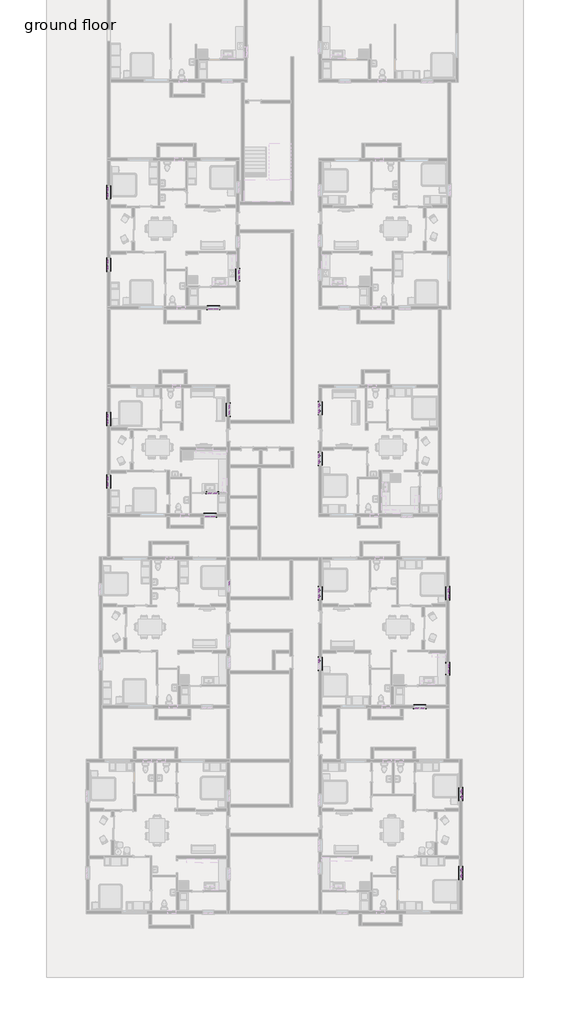
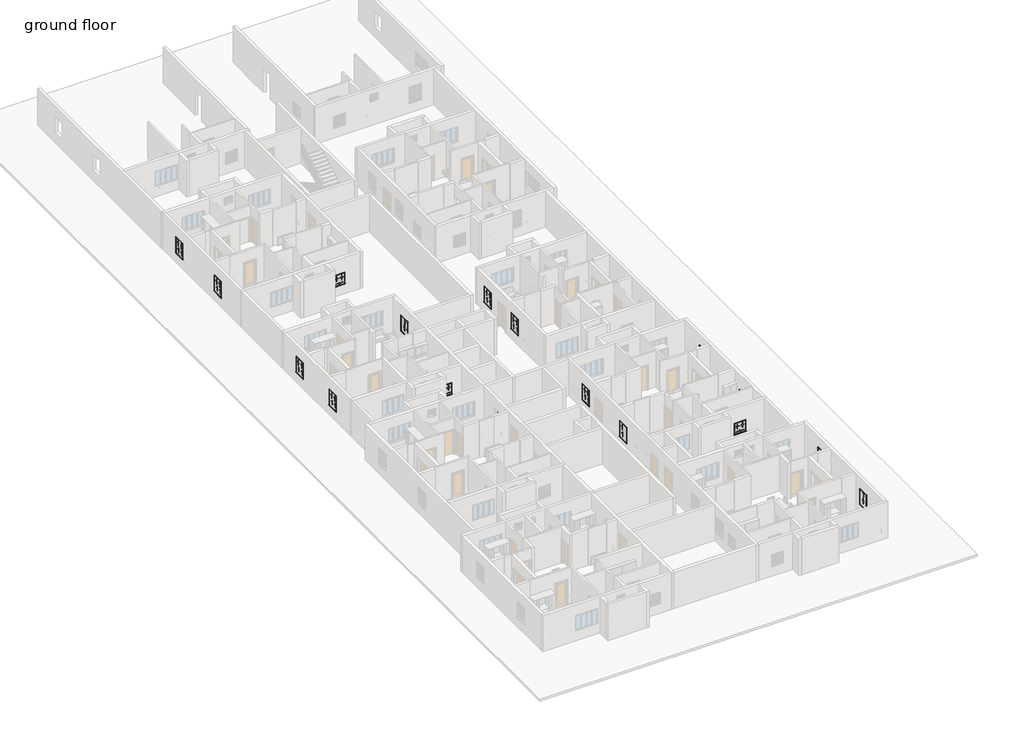
# One storey, part 15 of 16: 102 proxies.
"""IFC4 building model written with IfcOpenShell, lengths in millimetres."""

from ifc_helpers import new_model, si_unit, origin, place, context, project, spatial, transform, mapped, element, save
from components import muntin_pattern_2x2_muntin_pattern_2x2_cd1db81d, muntin_pattern_2x2_muntin_pattern_2x2_7c797e2d, muntin_pattern_2x2_muntin_pattern_2x2_78ce0566, muntin_pattern_2x2_muntin_pattern_2x2_27bf4e5b, muntin_pattern_2x2_muntin_pattern_2x2_8320156c, trim_window_exterior_flat_with_sill_fadbc092, trim_window_exterior_flat_with_sill_41619996, trim_window_interior_flat_picture_frame_db6fc9b7, trim_window_interior_flat_picture_frame_51c85655

model = new_model("IFC4")

# Units and contexts
model_context = context("Model", 3, world=origin())
ifc_project = project(units=[si_unit("LENGTHUNIT", "METRE", prefix="MILLI")], contexts=[model_context])

# Site, building, storey
site = spatial("IfcSite", under=ifc_project)
building = spatial("IfcBuilding", under=site)
storey = spatial("IfcBuildingStorey", under=building, Name="ground floor", Elevation=609.6)

# Proxies
placement = place(None, origin())
muntin_pattern_2x2_muntin_pattern_2x2_shape = muntin_pattern_2x2_muntin_pattern_2x2_cd1db81d(model_context)
element("IfcBuildingElementProxy", 1, Name="Muntin Pattern_2x2 : Muntin Pattern_2x2", ObjectType="Muntin Pattern_2x2 : Muntin Pattern_2x2", at=placement, inside=storey, context=model_context, shape_type="MappedRepresentation", body=[
    mapped(muntin_pattern_2x2_muntin_pattern_2x2_shape, transform((59391.4562819, 13667.0713152, 2206.625), x_axis=(0.0, 1.0, 0.0), y_axis=(-1.0, 0.0, 0.0), z_axis=(0.0, 0.0, 1.0))),
])
element("IfcBuildingElementProxy", 2, Name="Muntin Pattern_2x2 : Muntin Pattern_2x2", ObjectType="Muntin Pattern_2x2 : Muntin Pattern_2x2", at=placement, inside=storey, context=model_context, shape_type="MappedRepresentation", body=[
    mapped(muntin_pattern_2x2_muntin_pattern_2x2_shape, transform((59435.9062819, 13667.0713152, 1600.2), x_axis=(0.0, 1.0, 0.0), y_axis=(-1.0, 0.0, 0.0), z_axis=(0.0, 0.0, 1.0))),
])
element("IfcBuildingElementProxy", 3, Name="Muntin Pattern_2x2 : Muntin Pattern_2x2", ObjectType="Muntin Pattern_2x2 : Muntin Pattern_2x2", at=placement, inside=storey, context=model_context, shape_type="MappedRepresentation", body=[
    mapped(muntin_pattern_2x2_muntin_pattern_2x2_shape, transform((59391.4562819, 9780.8713152, 2206.625), x_axis=(0.0, 1.0, 0.0), y_axis=(-1.0, 0.0, 0.0), z_axis=(0.0, 0.0, 1.0))),
])
element("IfcBuildingElementProxy", 4, Name="Muntin Pattern_2x2 : Muntin Pattern_2x2", ObjectType="Muntin Pattern_2x2 : Muntin Pattern_2x2", at=placement, inside=storey, context=model_context, shape_type="MappedRepresentation", body=[
    mapped(muntin_pattern_2x2_muntin_pattern_2x2_shape, transform((59435.9062819, 9780.8713152, 1600.2), x_axis=(0.0, 1.0, 0.0), y_axis=(-1.0, 0.0, 0.0), z_axis=(0.0, 0.0, 1.0))),
])
element("IfcBuildingElementProxy", 5, Name="Muntin Pattern_2x2 : Muntin Pattern_2x2", ObjectType="Muntin Pattern_2x2 : Muntin Pattern_2x2", at=placement, inside=storey, context=model_context, shape_type="MappedRepresentation", body=[
    mapped(muntin_pattern_2x2_muntin_pattern_2x2_shape, transform((69329.2062819, -993.7176164, 2206.625), x_axis=(0.0, -1.0, 0.0), y_axis=(1.0, 0.0, 0.0), z_axis=(0.0, 0.0, 1.0))),
])
element("IfcBuildingElementProxy", 6, Name="Muntin Pattern_2x2 : Muntin Pattern_2x2", ObjectType="Muntin Pattern_2x2 : Muntin Pattern_2x2", at=placement, inside=storey, context=model_context, shape_type="MappedRepresentation", body=[
    mapped(muntin_pattern_2x2_muntin_pattern_2x2_shape, transform((69284.7562819, -993.7176164, 1600.2), x_axis=(0.0, -1.0, 0.0), y_axis=(1.0, 0.0, 0.0), z_axis=(0.0, 0.0, 1.0))),
])
element("IfcBuildingElementProxy", 7, Name="Muntin Pattern_2x2 : Muntin Pattern_2x2", ObjectType="Muntin Pattern_2x2 : Muntin Pattern_2x2", at=placement, inside=storey, context=model_context, shape_type="MappedRepresentation", body=[
    mapped(muntin_pattern_2x2_muntin_pattern_2x2_shape, transform((59391.4562819, -5948.3051164, 2206.625), x_axis=(0.0, 1.0, 0.0), y_axis=(-1.0, 0.0, 0.0), z_axis=(0.0, 0.0, 1.0))),
])
element("IfcBuildingElementProxy", 8, Name="Muntin Pattern_2x2 : Muntin Pattern_2x2", ObjectType="Muntin Pattern_2x2 : Muntin Pattern_2x2", at=placement, inside=storey, context=model_context, shape_type="MappedRepresentation", body=[
    mapped(muntin_pattern_2x2_muntin_pattern_2x2_shape, transform((59435.9062819, -5948.3051164, 1600.2), x_axis=(0.0, 1.0, 0.0), y_axis=(-1.0, 0.0, 0.0), z_axis=(0.0, 0.0, 1.0))),
])
element("IfcBuildingElementProxy", 9, Name="Muntin Pattern_2x2 : Muntin Pattern_2x2", ObjectType="Muntin Pattern_2x2 : Muntin Pattern_2x2", at=placement, inside=storey, context=model_context, shape_type="MappedRepresentation", body=[
    mapped(muntin_pattern_2x2_muntin_pattern_2x2_shape, transform((70332.5062819, -22465.6221086, 2206.625), x_axis=(0.0, -1.0, 0.0), y_axis=(1.0, 0.0, 0.0), z_axis=(0.0, 0.0, 1.0))),
])
element("IfcBuildingElementProxy", 10, Name="Muntin Pattern_2x2 : Muntin Pattern_2x2", ObjectType="Muntin Pattern_2x2 : Muntin Pattern_2x2", at=placement, inside=storey, context=model_context, shape_type="MappedRepresentation", body=[
    mapped(muntin_pattern_2x2_muntin_pattern_2x2_shape, transform((70288.0562819, -22465.6221086, 1600.2), x_axis=(0.0, -1.0, 0.0), y_axis=(1.0, 0.0, 0.0), z_axis=(0.0, 0.0, 1.0))),
])
element("IfcBuildingElementProxy", 11, Name="Muntin Pattern_2x2 : Muntin Pattern_2x2", ObjectType="Muntin Pattern_2x2 : Muntin Pattern_2x2", at=placement, inside=storey, context=model_context, shape_type="MappedRepresentation", body=[
    mapped(muntin_pattern_2x2_muntin_pattern_2x2_shape, transform((70332.5062819, -16407.8428409, 2206.625), x_axis=(0.0, -1.0, 0.0), y_axis=(1.0, 0.0, 0.0), z_axis=(0.0, 0.0, 1.0))),
])
element("IfcBuildingElementProxy", 12, Name="Muntin Pattern_2x2 : Muntin Pattern_2x2", ObjectType="Muntin Pattern_2x2 : Muntin Pattern_2x2", at=placement, inside=storey, context=model_context, shape_type="MappedRepresentation", body=[
    mapped(muntin_pattern_2x2_muntin_pattern_2x2_shape, transform((70288.0562819, -16407.8428409, 1600.2), x_axis=(0.0, -1.0, 0.0), y_axis=(1.0, 0.0, 0.0), z_axis=(0.0, 0.0, 1.0))),
])
element("IfcBuildingElementProxy", 13, Name="Muntin Pattern_2x2 : Muntin Pattern_2x2", ObjectType="Muntin Pattern_2x2 : Muntin Pattern_2x2", at=placement, inside=storey, context=model_context, shape_type="MappedRepresentation", body=[
    mapped(muntin_pattern_2x2_muntin_pattern_2x2_shape, transform((59391.4562819, -538.1051164, 2206.625), x_axis=(0.0, 1.0, 0.0), y_axis=(-1.0, 0.0, 0.0), z_axis=(0.0, 0.0, 1.0))),
])
element("IfcBuildingElementProxy", 14, Name="Muntin Pattern_2x2 : Muntin Pattern_2x2", ObjectType="Muntin Pattern_2x2 : Muntin Pattern_2x2", at=placement, inside=storey, context=model_context, shape_type="MappedRepresentation", body=[
    mapped(muntin_pattern_2x2_muntin_pattern_2x2_shape, transform((59435.9062819, -538.1051164, 1600.2), x_axis=(0.0, 1.0, 0.0), y_axis=(-1.0, 0.0, 0.0), z_axis=(0.0, 0.0, 1.0))),
])
element("IfcBuildingElementProxy", 15, Name="Muntin Pattern_2x2 : Muntin Pattern_2x2", ObjectType="Muntin Pattern_2x2 : Muntin Pattern_2x2", at=placement, inside=storey, context=model_context, shape_type="MappedRepresentation", body=[
    mapped(muntin_pattern_2x2_muntin_pattern_2x2_shape, transform((43176.551243, 8028.2713152, 2206.625), x_axis=(0.0, 1.0, 0.0), y_axis=(-1.0, 0.0, 0.0), z_axis=(0.0, 0.0, 1.0))),
])
element("IfcBuildingElementProxy", 16, Name="Muntin Pattern_2x2 : Muntin Pattern_2x2", ObjectType="Muntin Pattern_2x2 : Muntin Pattern_2x2", at=placement, inside=storey, context=model_context, shape_type="MappedRepresentation", body=[
    mapped(muntin_pattern_2x2_muntin_pattern_2x2_shape, transform((43221.001243, 8028.2713152, 1600.2), x_axis=(0.0, 1.0, 0.0), y_axis=(-1.0, 0.0, 0.0), z_axis=(0.0, 0.0, 1.0))),
])
element("IfcBuildingElementProxy", 17, Name="Muntin Pattern_2x2 : Muntin Pattern_2x2", ObjectType="Muntin Pattern_2x2 : Muntin Pattern_2x2", at=placement, inside=storey, context=model_context, shape_type="MappedRepresentation", body=[
    mapped(muntin_pattern_2x2_muntin_pattern_2x2_shape, transform((52504.701243, 13090.5355393, 2206.625), x_axis=(0.0, -1.0, 0.0), y_axis=(1.0, 0.0, 0.0), z_axis=(0.0, 0.0, 1.0))),
])
element("IfcBuildingElementProxy", 18, Name="Muntin Pattern_2x2 : Muntin Pattern_2x2", ObjectType="Muntin Pattern_2x2 : Muntin Pattern_2x2", at=placement, inside=storey, context=model_context, shape_type="MappedRepresentation", body=[
    mapped(muntin_pattern_2x2_muntin_pattern_2x2_shape, transform((52460.251243, 13090.5355393, 1600.2), x_axis=(0.0, -1.0, 0.0), y_axis=(1.0, 0.0, 0.0), z_axis=(0.0, 0.0, 1.0))),
])
element("IfcBuildingElementProxy", 19, Name="Muntin Pattern_2x2 : Muntin Pattern_2x2", ObjectType="Muntin Pattern_2x2 : Muntin Pattern_2x2", at=placement, inside=storey, context=model_context, shape_type="MappedRepresentation", body=[
    mapped(muntin_pattern_2x2_muntin_pattern_2x2_shape, transform((43176.551243, 12828.8713152, 2206.625), x_axis=(0.0, 1.0, 0.0), y_axis=(-1.0, 0.0, 0.0), z_axis=(0.0, 0.0, 1.0))),
])
element("IfcBuildingElementProxy", 20, Name="Muntin Pattern_2x2 : Muntin Pattern_2x2", ObjectType="Muntin Pattern_2x2 : Muntin Pattern_2x2", at=placement, inside=storey, context=model_context, shape_type="MappedRepresentation", body=[
    mapped(muntin_pattern_2x2_muntin_pattern_2x2_shape, transform((43221.001243, 12828.8713152, 1600.2), x_axis=(0.0, 1.0, 0.0), y_axis=(-1.0, 0.0, 0.0), z_axis=(0.0, 0.0, 1.0))),
])
element("IfcBuildingElementProxy", 21, Name="Muntin Pattern_2x2 : Muntin Pattern_2x2", ObjectType="Muntin Pattern_2x2 : Muntin Pattern_2x2", at=placement, inside=storey, context=model_context, shape_type="MappedRepresentation", body=[
    mapped(muntin_pattern_2x2_muntin_pattern_2x2_shape, transform((43176.551243, 24665.2713152, 2206.625), x_axis=(0.0, 1.0, 0.0), y_axis=(-1.0, 0.0, 0.0), z_axis=(0.0, 0.0, 1.0))),
])
element("IfcBuildingElementProxy", 22, Name="Muntin Pattern_2x2 : Muntin Pattern_2x2", ObjectType="Muntin Pattern_2x2 : Muntin Pattern_2x2", at=placement, inside=storey, context=model_context, shape_type="MappedRepresentation", body=[
    mapped(muntin_pattern_2x2_muntin_pattern_2x2_shape, transform((43221.001243, 24665.2713152, 1600.2), x_axis=(0.0, 1.0, 0.0), y_axis=(-1.0, 0.0, 0.0), z_axis=(0.0, 0.0, 1.0))),
])
element("IfcBuildingElementProxy", 23, Name="Muntin Pattern_2x2 : Muntin Pattern_2x2", ObjectType="Muntin Pattern_2x2 : Muntin Pattern_2x2", at=placement, inside=storey, context=model_context, shape_type="MappedRepresentation", body=[
    mapped(muntin_pattern_2x2_muntin_pattern_2x2_shape, transform((43176.551243, 30227.8713152, 2206.625), x_axis=(0.0, 1.0, 0.0), y_axis=(-1.0, 0.0, 0.0), z_axis=(0.0, 0.0, 1.0))),
])
element("IfcBuildingElementProxy", 24, Name="Muntin Pattern_2x2 : Muntin Pattern_2x2", ObjectType="Muntin Pattern_2x2 : Muntin Pattern_2x2", at=placement, inside=storey, context=model_context, shape_type="MappedRepresentation", body=[
    mapped(muntin_pattern_2x2_muntin_pattern_2x2_shape, transform((43221.001243, 30227.8713152, 1600.2), x_axis=(0.0, 1.0, 0.0), y_axis=(-1.0, 0.0, 0.0), z_axis=(0.0, 0.0, 1.0))),
])
muntin_pattern_2x2_muntin_pattern_2x2_2_shape = muntin_pattern_2x2_muntin_pattern_2x2_7c797e2d(model_context)
element("IfcBuildingElementProxy", 25, Name="Muntin Pattern_2x2 : Muntin Pattern_2x2", ObjectType="Muntin Pattern_2x2 : Muntin Pattern_2x2", at=placement, inside=storey, context=model_context, shape_type="MappedRepresentation", body=[
    mapped(muntin_pattern_2x2_muntin_pattern_2x2_2_shape, transform((59391.4562819, 13211.4588152, 2206.625), x_axis=(0.0, -1.0, 0.0), y_axis=(1.0, 0.0, 0.0), z_axis=(0.0, 0.0, 1.0))),
])
element("IfcBuildingElementProxy", 26, Name="Muntin Pattern_2x2 : Muntin Pattern_2x2", ObjectType="Muntin Pattern_2x2 : Muntin Pattern_2x2", at=placement, inside=storey, context=model_context, shape_type="MappedRepresentation", body=[
    mapped(muntin_pattern_2x2_muntin_pattern_2x2_2_shape, transform((59435.9062819, 13211.4588152, 1600.2), x_axis=(0.0, -1.0, 0.0), y_axis=(1.0, 0.0, 0.0), z_axis=(0.0, 0.0, 1.0))),
])
element("IfcBuildingElementProxy", 27, Name="Muntin Pattern_2x2 : Muntin Pattern_2x2", ObjectType="Muntin Pattern_2x2 : Muntin Pattern_2x2", at=placement, inside=storey, context=model_context, shape_type="MappedRepresentation", body=[
    mapped(muntin_pattern_2x2_muntin_pattern_2x2_2_shape, transform((59391.4562819, 9325.2588152, 2206.625), x_axis=(0.0, -1.0, 0.0), y_axis=(1.0, 0.0, 0.0), z_axis=(0.0, 0.0, 1.0))),
])
element("IfcBuildingElementProxy", 28, Name="Muntin Pattern_2x2 : Muntin Pattern_2x2", ObjectType="Muntin Pattern_2x2 : Muntin Pattern_2x2", at=placement, inside=storey, context=model_context, shape_type="MappedRepresentation", body=[
    mapped(muntin_pattern_2x2_muntin_pattern_2x2_2_shape, transform((59435.9062819, 9325.2588152, 1600.2), x_axis=(0.0, -1.0, 0.0), y_axis=(1.0, 0.0, 0.0), z_axis=(0.0, 0.0, 1.0))),
])
element("IfcBuildingElementProxy", 29, Name="Muntin Pattern_2x2 : Muntin Pattern_2x2", ObjectType="Muntin Pattern_2x2 : Muntin Pattern_2x2", at=placement, inside=storey, context=model_context, shape_type="MappedRepresentation", body=[
    mapped(muntin_pattern_2x2_muntin_pattern_2x2_2_shape, transform((69329.2062819, -538.1051164, 2206.625), x_axis=(0.0, 1.0, 0.0), y_axis=(-1.0, 0.0, 0.0), z_axis=(0.0, 0.0, 1.0))),
])
element("IfcBuildingElementProxy", 30, Name="Muntin Pattern_2x2 : Muntin Pattern_2x2", ObjectType="Muntin Pattern_2x2 : Muntin Pattern_2x2", at=placement, inside=storey, context=model_context, shape_type="MappedRepresentation", body=[
    mapped(muntin_pattern_2x2_muntin_pattern_2x2_2_shape, transform((69284.7562819, -538.1051164, 1600.2), x_axis=(0.0, 1.0, 0.0), y_axis=(-1.0, 0.0, 0.0), z_axis=(0.0, 0.0, 1.0))),
])
element("IfcBuildingElementProxy", 31, Name="Muntin Pattern_2x2 : Muntin Pattern_2x2", ObjectType="Muntin Pattern_2x2 : Muntin Pattern_2x2", at=placement, inside=storey, context=model_context, shape_type="MappedRepresentation", body=[
    mapped(muntin_pattern_2x2_muntin_pattern_2x2_2_shape, transform((70332.5062819, -22010.0096086, 2206.625), x_axis=(0.0, 1.0, 0.0), y_axis=(-1.0, 0.0, 0.0), z_axis=(0.0, 0.0, 1.0))),
])
element("IfcBuildingElementProxy", 32, Name="Muntin Pattern_2x2 : Muntin Pattern_2x2", ObjectType="Muntin Pattern_2x2 : Muntin Pattern_2x2", at=placement, inside=storey, context=model_context, shape_type="MappedRepresentation", body=[
    mapped(muntin_pattern_2x2_muntin_pattern_2x2_2_shape, transform((70288.0562819, -22010.0096086, 1600.2), x_axis=(0.0, 1.0, 0.0), y_axis=(-1.0, 0.0, 0.0), z_axis=(0.0, 0.0, 1.0))),
])
element("IfcBuildingElementProxy", 33, Name="Muntin Pattern_2x2 : Muntin Pattern_2x2", ObjectType="Muntin Pattern_2x2 : Muntin Pattern_2x2", at=placement, inside=storey, context=model_context, shape_type="MappedRepresentation", body=[
    mapped(muntin_pattern_2x2_muntin_pattern_2x2_2_shape, transform((70332.5062819, -15952.2303409, 2206.625), x_axis=(0.0, 1.0, 0.0), y_axis=(-1.0, 0.0, 0.0), z_axis=(0.0, 0.0, 1.0))),
])
element("IfcBuildingElementProxy", 34, Name="Muntin Pattern_2x2 : Muntin Pattern_2x2", ObjectType="Muntin Pattern_2x2 : Muntin Pattern_2x2", at=placement, inside=storey, context=model_context, shape_type="MappedRepresentation", body=[
    mapped(muntin_pattern_2x2_muntin_pattern_2x2_2_shape, transform((70288.0562819, -15952.2303409, 1600.2), x_axis=(0.0, 1.0, 0.0), y_axis=(-1.0, 0.0, 0.0), z_axis=(0.0, 0.0, 1.0))),
])
element("IfcBuildingElementProxy", 35, Name="Muntin Pattern_2x2 : Muntin Pattern_2x2", ObjectType="Muntin Pattern_2x2 : Muntin Pattern_2x2", at=placement, inside=storey, context=model_context, shape_type="MappedRepresentation", body=[
    mapped(muntin_pattern_2x2_muntin_pattern_2x2_2_shape, transform((59391.4562819, -993.7176164, 2206.625), x_axis=(0.0, -1.0, 0.0), y_axis=(1.0, 0.0, 0.0), z_axis=(0.0, 0.0, 1.0))),
])
element("IfcBuildingElementProxy", 36, Name="Muntin Pattern_2x2 : Muntin Pattern_2x2", ObjectType="Muntin Pattern_2x2 : Muntin Pattern_2x2", at=placement, inside=storey, context=model_context, shape_type="MappedRepresentation", body=[
    mapped(muntin_pattern_2x2_muntin_pattern_2x2_2_shape, transform((59435.9062819, -993.7176164, 1600.2), x_axis=(0.0, -1.0, 0.0), y_axis=(1.0, 0.0, 0.0), z_axis=(0.0, 0.0, 1.0))),
])
element("IfcBuildingElementProxy", 37, Name="Muntin Pattern_2x2 : Muntin Pattern_2x2", ObjectType="Muntin Pattern_2x2 : Muntin Pattern_2x2", at=placement, inside=storey, context=model_context, shape_type="MappedRepresentation", body=[
    mapped(muntin_pattern_2x2_muntin_pattern_2x2_2_shape, transform((43176.551243, 7572.6588152, 2206.625), x_axis=(0.0, -1.0, 0.0), y_axis=(1.0, 0.0, 0.0), z_axis=(0.0, 0.0, 1.0))),
])
element("IfcBuildingElementProxy", 38, Name="Muntin Pattern_2x2 : Muntin Pattern_2x2", ObjectType="Muntin Pattern_2x2 : Muntin Pattern_2x2", at=placement, inside=storey, context=model_context, shape_type="MappedRepresentation", body=[
    mapped(muntin_pattern_2x2_muntin_pattern_2x2_2_shape, transform((43221.001243, 7572.6588152, 1600.2), x_axis=(0.0, -1.0, 0.0), y_axis=(1.0, 0.0, 0.0), z_axis=(0.0, 0.0, 1.0))),
])
element("IfcBuildingElementProxy", 39, Name="Muntin Pattern_2x2 : Muntin Pattern_2x2", ObjectType="Muntin Pattern_2x2 : Muntin Pattern_2x2", at=placement, inside=storey, context=model_context, shape_type="MappedRepresentation", body=[
    mapped(muntin_pattern_2x2_muntin_pattern_2x2_2_shape, transform((52504.701243, 13546.1480393, 2206.625), x_axis=(0.0, 1.0, 0.0), y_axis=(-1.0, 0.0, 0.0), z_axis=(0.0, 0.0, 1.0))),
])
element("IfcBuildingElementProxy", 40, Name="Muntin Pattern_2x2 : Muntin Pattern_2x2", ObjectType="Muntin Pattern_2x2 : Muntin Pattern_2x2", at=placement, inside=storey, context=model_context, shape_type="MappedRepresentation", body=[
    mapped(muntin_pattern_2x2_muntin_pattern_2x2_2_shape, transform((52460.251243, 13546.1480393, 1600.2), x_axis=(0.0, 1.0, 0.0), y_axis=(-1.0, 0.0, 0.0), z_axis=(0.0, 0.0, 1.0))),
])
element("IfcBuildingElementProxy", 41, Name="Muntin Pattern_2x2 : Muntin Pattern_2x2", ObjectType="Muntin Pattern_2x2 : Muntin Pattern_2x2", at=placement, inside=storey, context=model_context, shape_type="MappedRepresentation", body=[
    mapped(muntin_pattern_2x2_muntin_pattern_2x2_2_shape, transform((43176.551243, 12373.2588152, 2206.625), x_axis=(0.0, -1.0, 0.0), y_axis=(1.0, 0.0, 0.0), z_axis=(0.0, 0.0, 1.0))),
])
element("IfcBuildingElementProxy", 42, Name="Muntin Pattern_2x2 : Muntin Pattern_2x2", ObjectType="Muntin Pattern_2x2 : Muntin Pattern_2x2", at=placement, inside=storey, context=model_context, shape_type="MappedRepresentation", body=[
    mapped(muntin_pattern_2x2_muntin_pattern_2x2_2_shape, transform((43221.001243, 12373.2588152, 1600.2), x_axis=(0.0, -1.0, 0.0), y_axis=(1.0, 0.0, 0.0), z_axis=(0.0, 0.0, 1.0))),
])
element("IfcBuildingElementProxy", 43, Name="Muntin Pattern_2x2 : Muntin Pattern_2x2", ObjectType="Muntin Pattern_2x2 : Muntin Pattern_2x2", at=placement, inside=storey, context=model_context, shape_type="MappedRepresentation", body=[
    mapped(muntin_pattern_2x2_muntin_pattern_2x2_2_shape, transform((43176.551243, 24209.6588152, 2206.625), x_axis=(0.0, -1.0, 0.0), y_axis=(1.0, 0.0, 0.0), z_axis=(0.0, 0.0, 1.0))),
])
element("IfcBuildingElementProxy", 44, Name="Muntin Pattern_2x2 : Muntin Pattern_2x2", ObjectType="Muntin Pattern_2x2 : Muntin Pattern_2x2", at=placement, inside=storey, context=model_context, shape_type="MappedRepresentation", body=[
    mapped(muntin_pattern_2x2_muntin_pattern_2x2_2_shape, transform((43221.001243, 24209.6588152, 1600.2), x_axis=(0.0, -1.0, 0.0), y_axis=(1.0, 0.0, 0.0), z_axis=(0.0, 0.0, 1.0))),
])
element("IfcBuildingElementProxy", 45, Name="Muntin Pattern_2x2 : Muntin Pattern_2x2", ObjectType="Muntin Pattern_2x2 : Muntin Pattern_2x2", at=placement, inside=storey, context=model_context, shape_type="MappedRepresentation", body=[
    mapped(muntin_pattern_2x2_muntin_pattern_2x2_2_shape, transform((43176.551243, 29772.2588152, 2206.625), x_axis=(0.0, -1.0, 0.0), y_axis=(1.0, 0.0, 0.0), z_axis=(0.0, 0.0, 1.0))),
])
element("IfcBuildingElementProxy", 46, Name="Muntin Pattern_2x2 : Muntin Pattern_2x2", ObjectType="Muntin Pattern_2x2 : Muntin Pattern_2x2", at=placement, inside=storey, context=model_context, shape_type="MappedRepresentation", body=[
    mapped(muntin_pattern_2x2_muntin_pattern_2x2_2_shape, transform((43221.001243, 29772.2588152, 1600.2), x_axis=(0.0, -1.0, 0.0), y_axis=(1.0, 0.0, 0.0), z_axis=(0.0, 0.0, 1.0))),
])
element("IfcBuildingElementProxy", 47, Name="Muntin Pattern_2x2 : Muntin Pattern_2x2", ObjectType="Muntin Pattern_2x2 : Muntin Pattern_2x2", at=placement, inside=storey, context=model_context, shape_type="MappedRepresentation", body=[
    mapped(muntin_pattern_2x2_muntin_pattern_2x2_2_shape, transform((52504.701243, 2.9653185, 2206.625), x_axis=(0.0, 1.0, 0.0), y_axis=(-1.0, 0.0, 0.0), z_axis=(0.0, 0.0, 1.0))),
])
element("IfcBuildingElementProxy", 48, Name="Muntin Pattern_2x2 : Muntin Pattern_2x2", ObjectType="Muntin Pattern_2x2 : Muntin Pattern_2x2", at=placement, inside=storey, context=model_context, shape_type="MappedRepresentation", body=[
    mapped(muntin_pattern_2x2_muntin_pattern_2x2_2_shape, transform((52460.251243, 2.9653185, 1600.2), x_axis=(0.0, 1.0, 0.0), y_axis=(-1.0, 0.0, 0.0), z_axis=(0.0, 0.0, 1.0))),
])
muntin_pattern_2x2_muntin_pattern_2x2_3_shape = muntin_pattern_2x2_muntin_pattern_2x2_78ce0566(model_context)
element("IfcBuildingElementProxy", 49, Name="Muntin Pattern_2x2 : Muntin Pattern_2x2", ObjectType="Muntin Pattern_2x2 : Muntin Pattern_2x2", at=placement, inside=storey, context=model_context, shape_type="MappedRepresentation", body=[
    mapped(muntin_pattern_2x2_muntin_pattern_2x2_3_shape, transform((69354.6062819, -6345.9738664, 1898.65), x_axis=(0.0, -1.0, 0.0), y_axis=(1.0, 0.0, 0.0), z_axis=(0.0, 0.0, 1.0))),
])
element("IfcBuildingElementProxy", 50, Name="Muntin Pattern_2x2 : Muntin Pattern_2x2", ObjectType="Muntin Pattern_2x2 : Muntin Pattern_2x2", at=placement, inside=storey, context=model_context, shape_type="MappedRepresentation", body=[
    mapped(muntin_pattern_2x2_muntin_pattern_2x2_3_shape, transform((67322.6640239, -9591.2174723, 1898.65), x_axis=(-1.0, 0.0, 0.0), y_axis=(0.0, -1.0, 0.0), z_axis=(0.0, 0.0, 1.0))),
])
element("IfcBuildingElementProxy", 51, Name="Muntin Pattern_2x2 : Muntin Pattern_2x2", ObjectType="Muntin Pattern_2x2 : Muntin Pattern_2x2", at=placement, inside=storey, context=model_context, shape_type="MappedRepresentation", body=[
    mapped(muntin_pattern_2x2_muntin_pattern_2x2_3_shape, transform((51229.408333, 5101.5968163, 1898.65), x_axis=(-1.0, 0.0, 0.0), y_axis=(0.0, -1.0, 0.0), z_axis=(0.0, 0.0, 1.0))),
])
element("IfcBuildingElementProxy", 52, Name="Muntin Pattern_2x2 : Muntin Pattern_2x2", ObjectType="Muntin Pattern_2x2 : Muntin Pattern_2x2", at=placement, inside=storey, context=model_context, shape_type="MappedRepresentation", body=[
    mapped(muntin_pattern_2x2_muntin_pattern_2x2_3_shape, transform((51417.263743, 6895.5900652, 1898.65), x_axis=(-1.0, 0.0, 0.0), y_axis=(0.0, -1.0, 0.0), z_axis=(0.0, 0.0, 1.0))),
])
element("IfcBuildingElementProxy", 53, Name="Muntin Pattern_2x2 : Muntin Pattern_2x2", ObjectType="Muntin Pattern_2x2 : Muntin Pattern_2x2", at=placement, inside=storey, context=model_context, shape_type="MappedRepresentation", body=[
    mapped(muntin_pattern_2x2_muntin_pattern_2x2_3_shape, transform((51489.2925, 21030.5522014, 1898.65), x_axis=(-1.0, 0.0, 0.0), y_axis=(0.0, -1.0, 0.0), z_axis=(0.0, 0.0, 1.0))),
])
element("IfcBuildingElementProxy", 54, Name="Muntin Pattern_2x2 : Muntin Pattern_2x2", ObjectType="Muntin Pattern_2x2 : Muntin Pattern_2x2", at=placement, inside=storey, context=model_context, shape_type="MappedRepresentation", body=[
    mapped(muntin_pattern_2x2_muntin_pattern_2x2_3_shape, transform((53254.001243, 23886.6025652, 1898.65), x_axis=(0.0, -1.0, 0.0), y_axis=(1.0, 0.0, 0.0), z_axis=(0.0, 0.0, 1.0))),
])
muntin_pattern_2x2_muntin_pattern_2x2_4_shape = muntin_pattern_2x2_muntin_pattern_2x2_27bf4e5b(model_context)
element("IfcBuildingElementProxy", 55, Name="Muntin Pattern_2x2 : Muntin Pattern_2x2", ObjectType="Muntin Pattern_2x2 : Muntin Pattern_2x2", at=placement, inside=storey, context=model_context, shape_type="MappedRepresentation", body=[
    mapped(muntin_pattern_2x2_muntin_pattern_2x2_4_shape, transform((69354.6062819, -6774.5988664, 1898.65), x_axis=(0.0, 1.0, 0.0), y_axis=(-1.0, 0.0, 0.0), z_axis=(0.0, 0.0, 1.0))),
])
element("IfcBuildingElementProxy", 56, Name="Muntin Pattern_2x2 : Muntin Pattern_2x2", ObjectType="Muntin Pattern_2x2 : Muntin Pattern_2x2", at=placement, inside=storey, context=model_context, shape_type="MappedRepresentation", body=[
    mapped(muntin_pattern_2x2_muntin_pattern_2x2_4_shape, transform((66894.0390239, -9591.2174723, 1898.65), x_axis=(1.0, 0.0, 0.0), y_axis=(0.0, 1.0, 0.0), z_axis=(0.0, 0.0, 1.0))),
])
element("IfcBuildingElementProxy", 57, Name="Muntin Pattern_2x2 : Muntin Pattern_2x2", ObjectType="Muntin Pattern_2x2 : Muntin Pattern_2x2", at=placement, inside=storey, context=model_context, shape_type="MappedRepresentation", body=[
    mapped(muntin_pattern_2x2_muntin_pattern_2x2_4_shape, transform((50800.783333, 5101.5968163, 1898.65), x_axis=(1.0, 0.0, 0.0), y_axis=(0.0, 1.0, 0.0), z_axis=(0.0, 0.0, 1.0))),
])
element("IfcBuildingElementProxy", 58, Name="Muntin Pattern_2x2 : Muntin Pattern_2x2", ObjectType="Muntin Pattern_2x2 : Muntin Pattern_2x2", at=placement, inside=storey, context=model_context, shape_type="MappedRepresentation", body=[
    mapped(muntin_pattern_2x2_muntin_pattern_2x2_4_shape, transform((50988.638743, 6895.5900652, 1898.65), x_axis=(1.0, 0.0, 0.0), y_axis=(0.0, 1.0, 0.0), z_axis=(0.0, 0.0, 1.0))),
])
element("IfcBuildingElementProxy", 59, Name="Muntin Pattern_2x2 : Muntin Pattern_2x2", ObjectType="Muntin Pattern_2x2 : Muntin Pattern_2x2", at=placement, inside=storey, context=model_context, shape_type="MappedRepresentation", body=[
    mapped(muntin_pattern_2x2_muntin_pattern_2x2_4_shape, transform((51060.6675, 21030.5522014, 1898.65), x_axis=(1.0, 0.0, 0.0), y_axis=(0.0, 1.0, 0.0), z_axis=(0.0, 0.0, 1.0))),
])
element("IfcBuildingElementProxy", 60, Name="Muntin Pattern_2x2 : Muntin Pattern_2x2", ObjectType="Muntin Pattern_2x2 : Muntin Pattern_2x2", at=placement, inside=storey, context=model_context, shape_type="MappedRepresentation", body=[
    mapped(muntin_pattern_2x2_muntin_pattern_2x2_4_shape, transform((53254.001243, 23457.9775652, 1898.65), x_axis=(0.0, 1.0, 0.0), y_axis=(-1.0, 0.0, 0.0), z_axis=(0.0, 0.0, 1.0))),
])
muntin_pattern_2x2_muntin_pattern_2x2_5_shape = muntin_pattern_2x2_muntin_pattern_2x2_8320156c(model_context)
element("IfcBuildingElementProxy", 61, Name="Muntin Pattern_2x2 : Muntin Pattern_2x2", ObjectType="Muntin Pattern_2x2 : Muntin Pattern_2x2", at=placement, inside=storey, context=model_context, shape_type="MappedRepresentation", body=[
    mapped(muntin_pattern_2x2_muntin_pattern_2x2_5_shape, transform((69354.6062819, -6560.2863664, 1593.85), x_axis=(0.0, 1.0, 0.0), y_axis=(-1.0, 0.0, 0.0), z_axis=(0.0, 0.0, 1.0))),
])
element("IfcBuildingElementProxy", 62, Name="Muntin Pattern_2x2 : Muntin Pattern_2x2", ObjectType="Muntin Pattern_2x2 : Muntin Pattern_2x2", at=placement, inside=storey, context=model_context, shape_type="MappedRepresentation", body=[
    mapped(muntin_pattern_2x2_muntin_pattern_2x2_5_shape, transform((67108.3515239, -9591.2174723, 1593.85), x_axis=(1.0, 0.0, 0.0), y_axis=(0.0, 1.0, 0.0), z_axis=(0.0, 0.0, 1.0))),
])
element("IfcBuildingElementProxy", 63, Name="Muntin Pattern_2x2 : Muntin Pattern_2x2", ObjectType="Muntin Pattern_2x2 : Muntin Pattern_2x2", at=placement, inside=storey, context=model_context, shape_type="MappedRepresentation", body=[
    mapped(muntin_pattern_2x2_muntin_pattern_2x2_5_shape, transform((51015.095833, 5101.5968163, 1593.85), x_axis=(1.0, 0.0, 0.0), y_axis=(0.0, 1.0, 0.0), z_axis=(0.0, 0.0, 1.0))),
])
element("IfcBuildingElementProxy", 64, Name="Muntin Pattern_2x2 : Muntin Pattern_2x2", ObjectType="Muntin Pattern_2x2 : Muntin Pattern_2x2", at=placement, inside=storey, context=model_context, shape_type="MappedRepresentation", body=[
    mapped(muntin_pattern_2x2_muntin_pattern_2x2_5_shape, transform((51202.951243, 6895.5900652, 1593.85), x_axis=(1.0, 0.0, 0.0), y_axis=(0.0, 1.0, 0.0), z_axis=(0.0, 0.0, 1.0))),
])
element("IfcBuildingElementProxy", 65, Name="Muntin Pattern_2x2 : Muntin Pattern_2x2", ObjectType="Muntin Pattern_2x2 : Muntin Pattern_2x2", at=placement, inside=storey, context=model_context, shape_type="MappedRepresentation", body=[
    mapped(muntin_pattern_2x2_muntin_pattern_2x2_5_shape, transform((51274.98, 21030.5522014, 1593.85), x_axis=(1.0, 0.0, 0.0), y_axis=(0.0, 1.0, 0.0), z_axis=(0.0, 0.0, 1.0))),
])
element("IfcBuildingElementProxy", 66, Name="Muntin Pattern_2x2 : Muntin Pattern_2x2", ObjectType="Muntin Pattern_2x2 : Muntin Pattern_2x2", at=placement, inside=storey, context=model_context, shape_type="MappedRepresentation", body=[
    mapped(muntin_pattern_2x2_muntin_pattern_2x2_5_shape, transform((53254.001243, 23672.2900652, 1593.85), x_axis=(0.0, 1.0, 0.0), y_axis=(-1.0, 0.0, 0.0), z_axis=(0.0, 0.0, 1.0))),
])
trim_window_exterior_flat_with_sill_shape = trim_window_exterior_flat_with_sill_fadbc092(model_context)
element("IfcBuildingElementProxy", 67, Name="Trim-Window-Exterior-Flat : with Sill", ObjectType="Trim-Window-Exterior-Flat : with Sill", at=placement, inside=storey, context=model_context, shape_type="MappedRepresentation", body=[
    mapped(trim_window_exterior_flat_with_sill_shape, transform((59356.5312819, 13439.2650652, 2844.8), x_axis=(0.0, -1.0, 0.0), y_axis=(0.0, 0.0, 1.0), z_axis=(-1.0, 0.0, 0.0))),
])
element("IfcBuildingElementProxy", 68, Name="Trim-Window-Exterior-Flat : with Sill", ObjectType="Trim-Window-Exterior-Flat : with Sill", at=placement, inside=storey, context=model_context, shape_type="MappedRepresentation", body=[
    mapped(trim_window_exterior_flat_with_sill_shape, transform((59356.5312819, 9553.0650652, 2844.8), x_axis=(0.0, -1.0, 0.0), y_axis=(0.0, 0.0, 1.0), z_axis=(-1.0, 0.0, 0.0))),
])
element("IfcBuildingElementProxy", 69, Name="Trim-Window-Exterior-Flat : with Sill", ObjectType="Trim-Window-Exterior-Flat : with Sill", at=placement, inside=storey, context=model_context, shape_type="MappedRepresentation", body=[
    mapped(trim_window_exterior_flat_with_sill_shape, transform((69364.1312819, -765.9113664, 2844.8), x_axis=(0.0, 1.0, 0.0), y_axis=(0.0, 0.0, 1.0), z_axis=(1.0, 0.0, 0.0))),
])
element("IfcBuildingElementProxy", 70, Name="Trim-Window-Exterior-Flat : with Sill", ObjectType="Trim-Window-Exterior-Flat : with Sill", at=placement, inside=storey, context=model_context, shape_type="MappedRepresentation", body=[
    mapped(trim_window_exterior_flat_with_sill_shape, transform((59356.5312819, -6176.1113664, 2844.8), x_axis=(0.0, -1.0, 0.0), y_axis=(0.0, 0.0, 1.0), z_axis=(-1.0, 0.0, 0.0))),
])
element("IfcBuildingElementProxy", 71, Name="Trim-Window-Exterior-Flat : with Sill", ObjectType="Trim-Window-Exterior-Flat : with Sill", at=placement, inside=storey, context=model_context, shape_type="MappedRepresentation", body=[
    mapped(trim_window_exterior_flat_with_sill_shape, transform((70367.4312819, -22237.8158586, 2844.8), x_axis=(0.0, 1.0, 0.0), y_axis=(0.0, 0.0, 1.0), z_axis=(1.0, 0.0, 0.0))),
])
element("IfcBuildingElementProxy", 72, Name="Trim-Window-Exterior-Flat : with Sill", ObjectType="Trim-Window-Exterior-Flat : with Sill", at=placement, inside=storey, context=model_context, shape_type="MappedRepresentation", body=[
    mapped(trim_window_exterior_flat_with_sill_shape, transform((70367.4312819, -16180.0365909, 2844.8), x_axis=(0.0, 1.0, 0.0), y_axis=(0.0, 0.0, 1.0), z_axis=(1.0, 0.0, 0.0))),
])
element("IfcBuildingElementProxy", 73, Name="Trim-Window-Exterior-Flat : with Sill", ObjectType="Trim-Window-Exterior-Flat : with Sill", at=placement, inside=storey, context=model_context, shape_type="MappedRepresentation", body=[
    mapped(trim_window_exterior_flat_with_sill_shape, transform((59356.5312819, -765.9113664, 2844.8), x_axis=(0.0, -1.0, 0.0), y_axis=(0.0, 0.0, 1.0), z_axis=(-1.0, 0.0, 0.0))),
])
element("IfcBuildingElementProxy", 74, Name="Trim-Window-Exterior-Flat : with Sill", ObjectType="Trim-Window-Exterior-Flat : with Sill", at=placement, inside=storey, context=model_context, shape_type="MappedRepresentation", body=[
    mapped(trim_window_exterior_flat_with_sill_shape, transform((43141.626243, 7800.4650652, 2844.8), x_axis=(0.0, -1.0, 0.0), y_axis=(0.0, 0.0, 1.0), z_axis=(-1.0, 0.0, 0.0))),
])
element("IfcBuildingElementProxy", 75, Name="Trim-Window-Exterior-Flat : with Sill", ObjectType="Trim-Window-Exterior-Flat : with Sill", at=placement, inside=storey, context=model_context, shape_type="MappedRepresentation", body=[
    mapped(trim_window_exterior_flat_with_sill_shape, transform((52539.626243, 13318.3417893, 2844.8), x_axis=(0.0, 1.0, 0.0), y_axis=(0.0, 0.0, 1.0), z_axis=(1.0, 0.0, 0.0))),
])
element("IfcBuildingElementProxy", 76, Name="Trim-Window-Exterior-Flat : with Sill", ObjectType="Trim-Window-Exterior-Flat : with Sill", at=placement, inside=storey, context=model_context, shape_type="MappedRepresentation", body=[
    mapped(trim_window_exterior_flat_with_sill_shape, transform((43141.626243, 12601.0650652, 2844.8), x_axis=(0.0, -1.0, 0.0), y_axis=(0.0, 0.0, 1.0), z_axis=(-1.0, 0.0, 0.0))),
])
element("IfcBuildingElementProxy", 77, Name="Trim-Window-Exterior-Flat : with Sill", ObjectType="Trim-Window-Exterior-Flat : with Sill", at=placement, inside=storey, context=model_context, shape_type="MappedRepresentation", body=[
    mapped(trim_window_exterior_flat_with_sill_shape, transform((43141.626243, 24437.4650652, 2844.8), x_axis=(0.0, -1.0, 0.0), y_axis=(0.0, 0.0, 1.0), z_axis=(-1.0, 0.0, 0.0))),
])
element("IfcBuildingElementProxy", 78, Name="Trim-Window-Exterior-Flat : with Sill", ObjectType="Trim-Window-Exterior-Flat : with Sill", at=placement, inside=storey, context=model_context, shape_type="MappedRepresentation", body=[
    mapped(trim_window_exterior_flat_with_sill_shape, transform((43141.626243, 30000.0650652, 2844.8), x_axis=(0.0, -1.0, 0.0), y_axis=(0.0, 0.0, 1.0), z_axis=(-1.0, 0.0, 0.0))),
])
trim_window_exterior_flat_with_sill_2_shape = trim_window_exterior_flat_with_sill_41619996(model_context)
element("IfcBuildingElementProxy", 79, Name="Trim-Window-Exterior-Flat : with Sill", ObjectType="Trim-Window-Exterior-Flat : with Sill", at=placement, inside=storey, context=model_context, shape_type="MappedRepresentation", body=[
    mapped(trim_window_exterior_flat_with_sill_2_shape, transform((69364.1312819, -6560.2863664, 2438.4), x_axis=(0.0, 1.0, 0.0), y_axis=(0.0, 0.0, 1.0), z_axis=(1.0, 0.0, 0.0))),
])
element("IfcBuildingElementProxy", 80, Name="Trim-Window-Exterior-Flat : with Sill", ObjectType="Trim-Window-Exterior-Flat : with Sill", at=placement, inside=storey, context=model_context, shape_type="MappedRepresentation", body=[
    mapped(trim_window_exterior_flat_with_sill_2_shape, transform((67108.3515239, -9600.7424723, 2438.4), x_axis=(1.0, 0.0, 0.0), y_axis=(0.0, 0.0, 1.0), z_axis=(0.0, -1.0, 0.0))),
])
element("IfcBuildingElementProxy", 81, Name="Trim-Window-Exterior-Flat : with Sill", ObjectType="Trim-Window-Exterior-Flat : with Sill", at=placement, inside=storey, context=model_context, shape_type="MappedRepresentation", body=[
    mapped(trim_window_exterior_flat_with_sill_2_shape, transform((51015.095833, 5092.0718163, 2438.4), x_axis=(1.0, 0.0, 0.0), y_axis=(0.0, 0.0, 1.0), z_axis=(0.0, -1.0, 0.0))),
])
element("IfcBuildingElementProxy", 82, Name="Trim-Window-Exterior-Flat : with Sill", ObjectType="Trim-Window-Exterior-Flat : with Sill", at=placement, inside=storey, context=model_context, shape_type="MappedRepresentation", body=[
    mapped(trim_window_exterior_flat_with_sill_2_shape, transform((51202.951243, 6886.0650652, 2438.4), x_axis=(1.0, 0.0, 0.0), y_axis=(0.0, 0.0, 1.0), z_axis=(0.0, -1.0, 0.0))),
])
element("IfcBuildingElementProxy", 83, Name="Trim-Window-Exterior-Flat : with Sill", ObjectType="Trim-Window-Exterior-Flat : with Sill", at=placement, inside=storey, context=model_context, shape_type="MappedRepresentation", body=[
    mapped(trim_window_exterior_flat_with_sill_2_shape, transform((51274.98, 21021.0272014, 2438.4), x_axis=(1.0, 0.0, 0.0), y_axis=(0.0, 0.0, 1.0), z_axis=(0.0, -1.0, 0.0))),
])
element("IfcBuildingElementProxy", 84, Name="Trim-Window-Exterior-Flat : with Sill", ObjectType="Trim-Window-Exterior-Flat : with Sill", at=placement, inside=storey, context=model_context, shape_type="MappedRepresentation", body=[
    mapped(trim_window_exterior_flat_with_sill_2_shape, transform((53263.526243, 23672.2900652, 2438.4), x_axis=(0.0, 1.0, 0.0), y_axis=(0.0, 0.0, 1.0), z_axis=(1.0, 0.0, 0.0))),
])
trim_window_interior_flat_picture_frame_shape = trim_window_interior_flat_picture_frame_db6fc9b7(model_context)
element("IfcBuildingElementProxy", 85, Name="Trim-Window-Interior-Flat : Picture Frame", ObjectType="Trim-Window-Interior-Flat : Picture Frame", at=placement, inside=storey, context=model_context, shape_type="MappedRepresentation", body=[
    mapped(trim_window_interior_flat_picture_frame_shape, transform((59585.1312819, 13439.2650652, 2844.8), x_axis=(0.0, 1.0, 0.0), y_axis=(0.0, 0.0, 1.0), z_axis=(1.0, 0.0, 0.0))),
])
element("IfcBuildingElementProxy", 86, Name="Trim-Window-Interior-Flat : Picture Frame", ObjectType="Trim-Window-Interior-Flat : Picture Frame", at=placement, inside=storey, context=model_context, shape_type="MappedRepresentation", body=[
    mapped(trim_window_interior_flat_picture_frame_shape, transform((59585.1312819, 9553.0650652, 2844.8), x_axis=(0.0, 1.0, 0.0), y_axis=(0.0, 0.0, 1.0), z_axis=(1.0, 0.0, 0.0))),
])
element("IfcBuildingElementProxy", 87, Name="Trim-Window-Interior-Flat : Picture Frame", ObjectType="Trim-Window-Interior-Flat : Picture Frame", at=placement, inside=storey, context=model_context, shape_type="MappedRepresentation", body=[
    mapped(trim_window_interior_flat_picture_frame_shape, transform((69135.5312819, -765.9113664, 2844.8), x_axis=(0.0, -1.0, 0.0), y_axis=(0.0, 0.0, 1.0), z_axis=(-1.0, 0.0, 0.0))),
])
element("IfcBuildingElementProxy", 88, Name="Trim-Window-Interior-Flat : Picture Frame", ObjectType="Trim-Window-Interior-Flat : Picture Frame", at=placement, inside=storey, context=model_context, shape_type="MappedRepresentation", body=[
    mapped(trim_window_interior_flat_picture_frame_shape, transform((59585.1312819, -6176.1113664, 2844.8), x_axis=(0.0, 1.0, 0.0), y_axis=(0.0, 0.0, 1.0), z_axis=(1.0, 0.0, 0.0))),
])
element("IfcBuildingElementProxy", 89, Name="Trim-Window-Interior-Flat : Picture Frame", ObjectType="Trim-Window-Interior-Flat : Picture Frame", at=placement, inside=storey, context=model_context, shape_type="MappedRepresentation", body=[
    mapped(trim_window_interior_flat_picture_frame_shape, transform((70138.8312819, -22237.8158586, 2844.8), x_axis=(0.0, -1.0, 0.0), y_axis=(0.0, 0.0, 1.0), z_axis=(-1.0, 0.0, 0.0))),
])
element("IfcBuildingElementProxy", 90, Name="Trim-Window-Interior-Flat : Picture Frame", ObjectType="Trim-Window-Interior-Flat : Picture Frame", at=placement, inside=storey, context=model_context, shape_type="MappedRepresentation", body=[
    mapped(trim_window_interior_flat_picture_frame_shape, transform((70138.8312819, -16180.0365909, 2844.8), x_axis=(0.0, -1.0, 0.0), y_axis=(0.0, 0.0, 1.0), z_axis=(-1.0, 0.0, 0.0))),
])
element("IfcBuildingElementProxy", 91, Name="Trim-Window-Interior-Flat : Picture Frame", ObjectType="Trim-Window-Interior-Flat : Picture Frame", at=placement, inside=storey, context=model_context, shape_type="MappedRepresentation", body=[
    mapped(trim_window_interior_flat_picture_frame_shape, transform((59585.1312819, -765.9113664, 2844.8), x_axis=(0.0, 1.0, 0.0), y_axis=(0.0, 0.0, 1.0), z_axis=(1.0, 0.0, 0.0))),
])
element("IfcBuildingElementProxy", 92, Name="Trim-Window-Interior-Flat : Picture Frame", ObjectType="Trim-Window-Interior-Flat : Picture Frame", at=placement, inside=storey, context=model_context, shape_type="MappedRepresentation", body=[
    mapped(trim_window_interior_flat_picture_frame_shape, transform((43370.226243, 7800.4650652, 2844.8), x_axis=(0.0, 1.0, 0.0), y_axis=(0.0, 0.0, 1.0), z_axis=(1.0, 0.0, 0.0))),
])
element("IfcBuildingElementProxy", 93, Name="Trim-Window-Interior-Flat : Picture Frame", ObjectType="Trim-Window-Interior-Flat : Picture Frame", at=placement, inside=storey, context=model_context, shape_type="MappedRepresentation", body=[
    mapped(trim_window_interior_flat_picture_frame_shape, transform((52311.026243, 13318.3417893, 2844.8), x_axis=(0.0, -1.0, 0.0), y_axis=(0.0, 0.0, 1.0), z_axis=(-1.0, 0.0, 0.0))),
])
element("IfcBuildingElementProxy", 94, Name="Trim-Window-Interior-Flat : Picture Frame", ObjectType="Trim-Window-Interior-Flat : Picture Frame", at=placement, inside=storey, context=model_context, shape_type="MappedRepresentation", body=[
    mapped(trim_window_interior_flat_picture_frame_shape, transform((43370.226243, 12601.0650652, 2844.8), x_axis=(0.0, 1.0, 0.0), y_axis=(0.0, 0.0, 1.0), z_axis=(1.0, 0.0, 0.0))),
])
element("IfcBuildingElementProxy", 95, Name="Trim-Window-Interior-Flat : Picture Frame", ObjectType="Trim-Window-Interior-Flat : Picture Frame", at=placement, inside=storey, context=model_context, shape_type="MappedRepresentation", body=[
    mapped(trim_window_interior_flat_picture_frame_shape, transform((43370.226243, 24437.4650652, 2844.8), x_axis=(0.0, 1.0, 0.0), y_axis=(0.0, 0.0, 1.0), z_axis=(1.0, 0.0, 0.0))),
])
element("IfcBuildingElementProxy", 96, Name="Trim-Window-Interior-Flat : Picture Frame", ObjectType="Trim-Window-Interior-Flat : Picture Frame", at=placement, inside=storey, context=model_context, shape_type="MappedRepresentation", body=[
    mapped(trim_window_interior_flat_picture_frame_shape, transform((43370.226243, 30000.0650652, 2844.8), x_axis=(0.0, 1.0, 0.0), y_axis=(0.0, 0.0, 1.0), z_axis=(1.0, 0.0, 0.0))),
])
trim_window_interior_flat_picture_frame_2_shape = trim_window_interior_flat_picture_frame_51c85655(model_context)
element("IfcBuildingElementProxy", 97, Name="Trim-Window-Interior-Flat : Picture Frame", ObjectType="Trim-Window-Interior-Flat : Picture Frame", at=placement, inside=storey, context=model_context, shape_type="MappedRepresentation", body=[
    mapped(trim_window_interior_flat_picture_frame_2_shape, transform((69135.5312819, -6560.2863664, 2438.4), x_axis=(0.0, -1.0, 0.0), y_axis=(0.0, 0.0, 1.0), z_axis=(-1.0, 0.0, 0.0))),
])
element("IfcBuildingElementProxy", 98, Name="Trim-Window-Interior-Flat : Picture Frame", ObjectType="Trim-Window-Interior-Flat : Picture Frame", at=placement, inside=storey, context=model_context, shape_type="MappedRepresentation", body=[
    mapped(trim_window_interior_flat_picture_frame_2_shape, transform((67108.3515239, -9372.1424723, 2438.4), x_axis=(-1.0, 0.0, 0.0), y_axis=(0.0, 0.0, 1.0), z_axis=(0.0, 1.0, 0.0))),
])
element("IfcBuildingElementProxy", 99, Name="Trim-Window-Interior-Flat : Picture Frame", ObjectType="Trim-Window-Interior-Flat : Picture Frame", at=placement, inside=storey, context=model_context, shape_type="MappedRepresentation", body=[
    mapped(trim_window_interior_flat_picture_frame_2_shape, transform((51015.095833, 5320.6718163, 2438.4), x_axis=(-1.0, 0.0, 0.0), y_axis=(0.0, 0.0, 1.0), z_axis=(0.0, 1.0, 0.0))),
])
element("IfcBuildingElementProxy", 100, Name="Trim-Window-Interior-Flat : Picture Frame", ObjectType="Trim-Window-Interior-Flat : Picture Frame", at=placement, inside=storey, context=model_context, shape_type="MappedRepresentation", body=[
    mapped(trim_window_interior_flat_picture_frame_2_shape, transform((51202.951243, 7000.3650652, 2438.4), x_axis=(-1.0, 0.0, 0.0), y_axis=(0.0, 0.0, 1.0), z_axis=(0.0, 1.0, 0.0))),
])
element("IfcBuildingElementProxy", 101, Name="Trim-Window-Interior-Flat : Picture Frame", ObjectType="Trim-Window-Interior-Flat : Picture Frame", at=placement, inside=storey, context=model_context, shape_type="MappedRepresentation", body=[
    mapped(trim_window_interior_flat_picture_frame_2_shape, transform((51274.98, 21249.6272014, 2438.4), x_axis=(-1.0, 0.0, 0.0), y_axis=(0.0, 0.0, 1.0), z_axis=(0.0, 1.0, 0.0))),
])
element("IfcBuildingElementProxy", 102, Name="Trim-Window-Interior-Flat : Picture Frame", ObjectType="Trim-Window-Interior-Flat : Picture Frame", at=placement, inside=storey, context=model_context, shape_type="MappedRepresentation", body=[
    mapped(trim_window_interior_flat_picture_frame_2_shape, transform((53034.926243, 23672.2900652, 2438.4), x_axis=(0.0, -1.0, 0.0), y_axis=(0.0, 0.0, 1.0), z_axis=(-1.0, 0.0, 0.0))),
])

save(model, "model.ifc")

# Revit data of these elements
# Type "Muntin Pattern_2x2 : Muntin Pattern_2x2"
#   Width [instance default] = 4' - 0"
#   Thickness = 0' - 0 1/2"
#   Height [instance default] = 4' - 0"
#   Distance = 0' - 0 3/4"
#   Interior Material [instance default] = none
#   Exterior Material [instance default] = none
#   Default Elevation = 0
# Type "Trim-Window-Exterior-Flat : with Sill"
#   Trim Width = 0' - 2 1/4"
#   Trim Thickness_Picture Frame = 0' - 1 1/4"
#   Trim Thickness_with Sill = 0' - 0 3/4"
#   Sill Thickness = 0' - 1 1/4"
#   Opening Width [instance default] = 2' - 0"
#   Opening Height [instance default] = 3' - 0"
#   Default Elevation = 4' - 0"
#   Sill = yes
#   Picture Frame = no
#   Trim Material [instance default] = none
# Type "Trim-Window-Interior-Flat : Picture Frame"
#   Trim Thickness_Picture Frame = 0' - 1 1/4"
#   Trim Width = 0' - 2 1/4"
#   Trim Thickness_with Sill = 0' - 0 3/4"
#   Sill Thickness = 0' - 1 1/4"
#   Opening Width [instance default] = 2' - 0"
#   Opening Height [instance default] = 3' - 0"
#   Default Elevation = 4' - 0"
#   Sill = no
#   Picture Frame = yes
#   Trim Material [instance default] = none
# Elements 1, 2, 3, 4, 5, 6, 7, 8, 9, 10, 11, 12, 13, 14, 15, 16, 17, 18, 19, 20, 21, 22, 23, 24, 25, 26, 27, 28, 29, 30, 31, 32, 33, 34, 35, 36, 37, 38, 39, 40, 41, 42, 43, 44, 45, 46, 47, 48 (IfcBuildingElementProxy, "Muntin Pattern_2x2 : Muntin Pattern_2x2")
#   Width = 1' - 0 1/16"
#   Height = 1' - 10 1/8"
#   Interior Material = Wood - Stained
#   Exterior Material = Clad - White
#   Phase Created = New Construction
#   Materials on its faces: "Clad - White", "Wood - Stained"
# Elements 49, 50, 51, 52, 53, 54, 55, 56, 57, 58, 59, 60 (IfcBuildingElementProxy, "Muntin Pattern_2x2 : Muntin Pattern_2x2")
#   Width = 0' - 11 5/8"
#   Height = 1' - 6 1/2"
#   Interior Material = Wood - Stained
#   Exterior Material = Clad - White
#   Phase Created = New Construction
#   Materials on its faces: "Clad - White", "Wood - Stained"
# Elements 61, 62, 63, 64, 65, 66 (IfcBuildingElementProxy, "Muntin Pattern_2x2 : Muntin Pattern_2x2")
#   Width = 2' - 4 1/2"
#   Height = 0' - 6 1/2"
#   Interior Material = Wood - Stained
#   Exterior Material = Clad - White
#   Phase Created = New Construction
#   Materials on its faces: "Clad - White", "Wood - Stained"
# Elements 67, 68, 69, 70, 71, 72, 73, 74, 75, 76, 77, 78 (IfcBuildingElementProxy, "Trim-Window-Exterior-Flat : with Sill")
#   Opening Width = 3' - 0"
#   Opening Height = 4' - 4"
#   Trim Material = Clad - White
#   Phase Created = New Construction
#   Materials on its faces: "Clad - White"
# Elements 79, 80, 81, 82, 83, 84 (IfcBuildingElementProxy, "Trim-Window-Exterior-Flat : with Sill")
#   Opening Width = 2' - 10"
#   Opening Height = 3' - 0"
#   Trim Material = Clad - White
#   Phase Created = New Construction
#   Materials on its faces: "Clad - White"
# Elements 85, 86, 87, 88, 89, 90, 91, 92, 93, 94, 95, 96 (IfcBuildingElementProxy, "Trim-Window-Interior-Flat : Picture Frame")
#   Opening Width = 3' - 0"
#   Opening Height = 4' - 4"
#   Trim Material = Wood - Stained
#   Phase Created = New Construction
#   Materials on its faces: "Wood - Stained"
# Elements 97, 98, 99, 100, 101, 102 (IfcBuildingElementProxy, "Trim-Window-Interior-Flat : Picture Frame")
#   Opening Width = 2' - 10"
#   Opening Height = 3' - 0"
#   Trim Material = Wood - Stained
#   Phase Created = New Construction
#   Materials on its faces: "Wood - Stained"
# Materials
#   "Clad - White": class "Wood", colour RGB 242 242 238, transparency 0, Cost = 0
#   "Wood - Stained": class "Wood", colour RGB 224 178 126, transparency 0, Cost = 0
